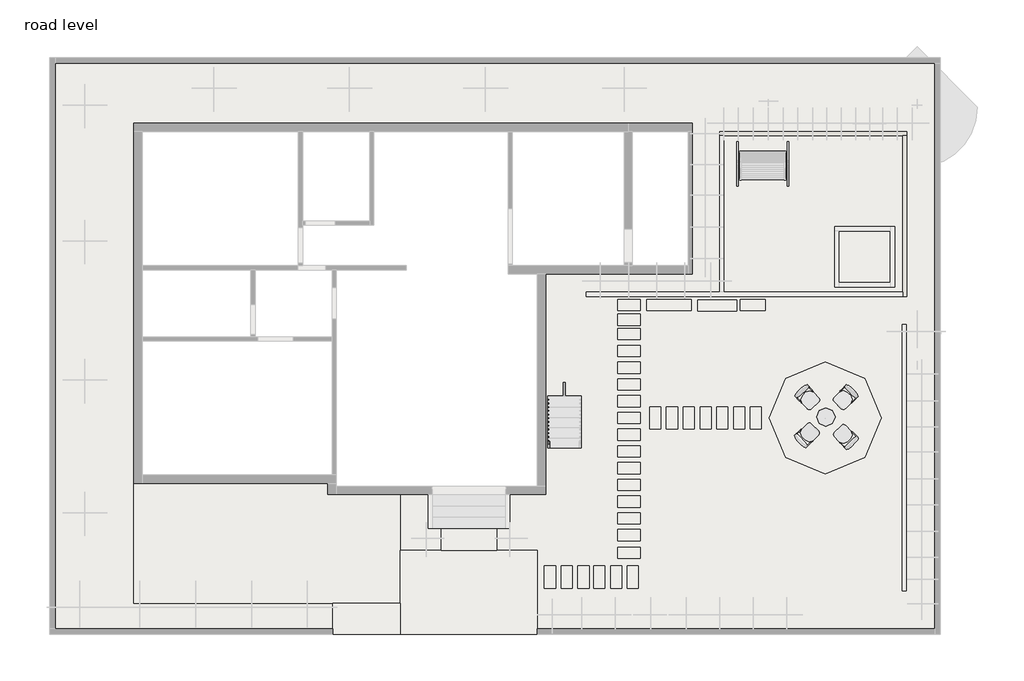
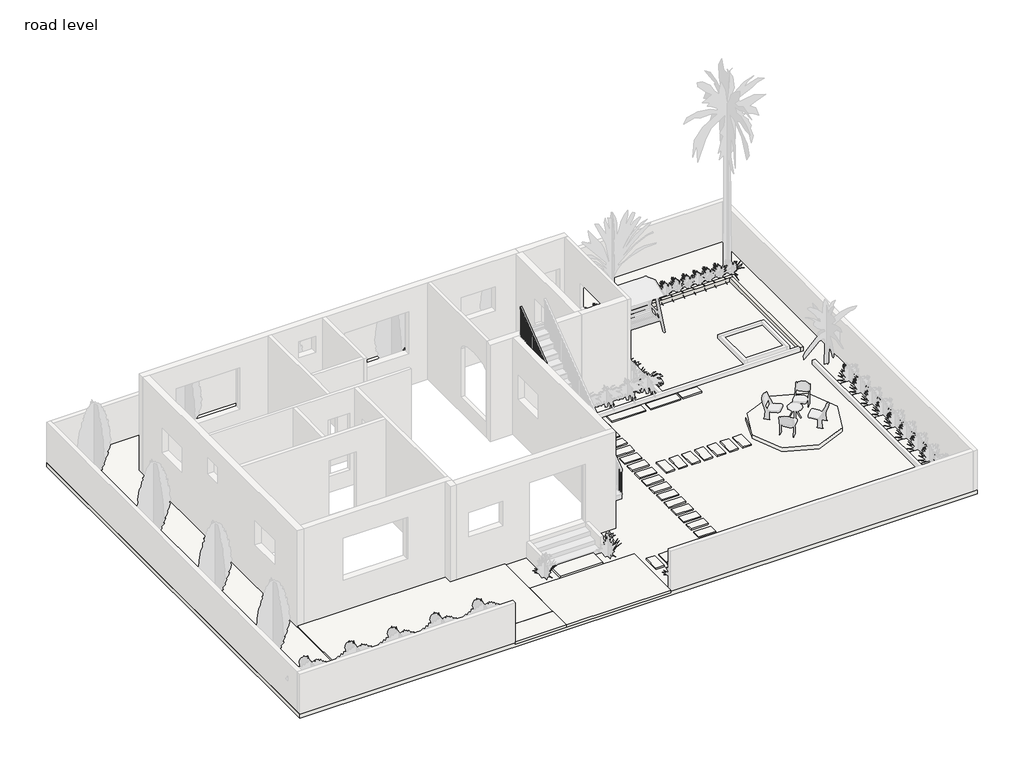
# One storey, part 2 of 3: 12 slabs, 2 walls, 1 railing.
"""IFC4 building model written with IfcOpenShell, lengths in millimetres."""

from ifc_helpers import new_model, si_unit, point, frame, frame_2d, origin, origin_with_axes, place, context, project, spatial, polyline, circle_curve, trimmed, segment, composite_curve, outline, extrude, faceted_brep, element, save

model = new_model("IFC4")

# Units and contexts
model_context = context("Model", 3, world=origin())
ifc_project = project(units=[si_unit("LENGTHUNIT", "METRE", prefix="MILLI")], contexts=[model_context])

# Site, building, storey
site = spatial("IfcSite", under=ifc_project)
building = spatial("IfcBuilding", under=site)
storey = spatial("IfcBuildingStorey", under=building, Name="road level", Elevation=0.0)

# Railing
placement = place(None, origin())
element("IfcRailing", 1, ObjectType="Handrail - Rectangular", at=placement, inside=storey, context=model_context, shape_type="SweptSolid", body=[
    extrude(outline(polyline([(3730.2992417, 1062.3350139), (3730.2992417, 1126.0666667), (8480.0992417, 4724.4), (8480.0992417, 4660.6683472), (3730.2992417, 1062.3350139)])), frame((-6743.6917413, 0.0, 0.0), z_axis=(1.0, 0.0, 0.0), x_axis=(0.0, 1.0, 0.0)), (0.0, 0.0, 1.0), 50.8),
    extrude(outline(polyline([(8413.4242417, 4610.1569836), (8413.4242417, 3598.3333333), (8394.3742417, 3598.3333333), (8394.3742417, 4595.7251654), (8413.4242417, 4610.1569836)])), frame((-6727.8167413, 0.0, 0.0), z_axis=(1.0, 0.0, 0.0), x_axis=(0.0, 1.0, 0.0)), (0.0, 0.0, 1.0), 19.05),
    extrude(outline(polyline([(8311.8242417, 4533.1872866), (8311.8242417, 3598.3333333), (8292.7742417, 3598.3333333), (8292.7742417, 4518.7554685), (8311.8242417, 4533.1872866)])), frame((-6727.8167413, 0.0, 0.0), z_axis=(1.0, 0.0, 0.0), x_axis=(0.0, 1.0, 0.0)), (0.0, 0.0, 1.0), 19.05),
    extrude(outline(polyline([(8210.2242417, 4456.2175897), (8210.2242417, 3598.3333333), (8191.1742417, 3598.3333333), (8191.1742417, 4441.7857715), (8210.2242417, 4456.2175897)])), frame((-6727.8167413, 0.0, 0.0), z_axis=(1.0, 0.0, 0.0), x_axis=(0.0, 1.0, 0.0)), (0.0, 0.0, 1.0), 19.05),
    extrude(outline(polyline([(8108.6242417, 4379.2478927), (8108.6242417, 3386.6666667), (8089.5742417, 3386.6666667), (8089.5742417, 4364.8160745), (8108.6242417, 4379.2478927)])), frame((-6727.8167413, 0.0, 0.0), z_axis=(1.0, 0.0, 0.0), x_axis=(0.0, 1.0, 0.0)), (0.0, 0.0, 1.0), 19.05),
    extrude(outline(polyline([(8007.0242417, 4302.2781957), (8007.0242417, 3386.6666667), (7987.9742417, 3386.6666667), (7987.9742417, 4287.8463775), (8007.0242417, 4302.2781957)])), frame((-6727.8167413, 0.0, 0.0), z_axis=(1.0, 0.0, 0.0), x_axis=(0.0, 1.0, 0.0)), (0.0, 0.0, 1.0), 19.05),
    extrude(outline(polyline([(7905.4242417, 4225.3084988), (7905.4242417, 3175.0), (7886.3742417, 3175.0), (7886.3742417, 4210.8766806), (7905.4242417, 4225.3084988)])), frame((-6727.8167413, 0.0, 0.0), z_axis=(1.0, 0.0, 0.0), x_axis=(0.0, 1.0, 0.0)), (0.0, 0.0, 1.0), 19.05),
    extrude(outline(polyline([(7803.8242417, 4148.3388018), (7803.8242417, 3175.0), (7784.7742417, 3175.0), (7784.7742417, 4133.9069836), (7803.8242417, 4148.3388018)])), frame((-6727.8167413, 0.0, 0.0), z_axis=(1.0, 0.0, 0.0), x_axis=(0.0, 1.0, 0.0)), (0.0, 0.0, 1.0), 19.05),
    extrude(outline(polyline([(7702.2242417, 4071.3691048), (7702.2242417, 3175.0), (7683.1742417, 3175.0), (7683.1742417, 4056.9372866), (7702.2242417, 4071.3691048)])), frame((-6727.8167413, 0.0, 0.0), z_axis=(1.0, 0.0, 0.0), x_axis=(0.0, 1.0, 0.0)), (0.0, 0.0, 1.0), 19.05),
    extrude(outline(polyline([(7600.6242417, 3994.3994079), (7600.6242417, 2963.3333333), (7581.5742417, 2963.3333333), (7581.5742417, 3979.9675897), (7600.6242417, 3994.3994079)])), frame((-6727.8167413, 0.0, 0.0), z_axis=(1.0, 0.0, 0.0), x_axis=(0.0, 1.0, 0.0)), (0.0, 0.0, 1.0), 19.05),
    extrude(outline(polyline([(7499.0242417, 3917.4297109), (7499.0242417, 2963.3333333), (7479.9742417, 2963.3333333), (7479.9742417, 3902.9978927), (7499.0242417, 3917.4297109)])), frame((-6727.8167413, 0.0, 0.0), z_axis=(1.0, 0.0, 0.0), x_axis=(0.0, 1.0, 0.0)), (0.0, 0.0, 1.0), 19.05),
    extrude(outline(polyline([(7397.4242417, 3840.4600139), (7397.4242417, 2963.3333333), (7378.3742417, 2963.3333333), (7378.3742417, 3826.0281957), (7397.4242417, 3840.4600139)])), frame((-6727.8167413, 0.0, 0.0), z_axis=(1.0, 0.0, 0.0), x_axis=(0.0, 1.0, 0.0)), (0.0, 0.0, 1.0), 19.05),
    extrude(outline(polyline([(7295.8242417, 3763.4903169), (7295.8242417, 2751.6666667), (7276.7742417, 2751.6666667), (7276.7742417, 3749.0584988), (7295.8242417, 3763.4903169)])), frame((-6727.8167413, 0.0, 0.0), z_axis=(1.0, 0.0, 0.0), x_axis=(0.0, 1.0, 0.0)), (0.0, 0.0, 1.0), 19.05),
    extrude(outline(polyline([(7194.2242417, 3686.52062), (7194.2242417, 2751.6666667), (7175.1742417, 2751.6666667), (7175.1742417, 3672.0888018), (7194.2242417, 3686.52062)])), frame((-6727.8167413, 0.0, 0.0), z_axis=(1.0, 0.0, 0.0), x_axis=(0.0, 1.0, 0.0)), (0.0, 0.0, 1.0), 19.05),
    extrude(outline(polyline([(7092.6242417, 3609.550923), (7092.6242417, 2751.6666667), (7073.5742417, 2751.6666667), (7073.5742417, 3595.1191048), (7092.6242417, 3609.550923)])), frame((-6727.8167413, 0.0, 0.0), z_axis=(1.0, 0.0, 0.0), x_axis=(0.0, 1.0, 0.0)), (0.0, 0.0, 1.0), 19.05),
    extrude(outline(polyline([(6991.0242417, 3532.581226), (6991.0242417, 2540.0), (6971.9742417, 2540.0), (6971.9742417, 3518.1494079), (6991.0242417, 3532.581226)])), frame((-6727.8167413, 0.0, 0.0), z_axis=(1.0, 0.0, 0.0), x_axis=(0.0, 1.0, 0.0)), (0.0, 0.0, 1.0), 19.05),
    extrude(outline(polyline([(6889.4242417, 3455.6115291), (6889.4242417, 2540.0), (6870.3742417, 2540.0), (6870.3742417, 3441.1797109), (6889.4242417, 3455.6115291)])), frame((-6727.8167413, 0.0, 0.0), z_axis=(1.0, 0.0, 0.0), x_axis=(0.0, 1.0, 0.0)), (0.0, 0.0, 1.0), 19.05),
    extrude(outline(polyline([(6787.8242417, 3378.6418321), (6787.8242417, 2328.3333333), (6768.7742417, 2328.3333333), (6768.7742417, 3364.2100139), (6787.8242417, 3378.6418321)])), frame((-6727.8167413, 0.0, 0.0), z_axis=(1.0, 0.0, 0.0), x_axis=(0.0, 1.0, 0.0)), (0.0, 0.0, 1.0), 19.05),
    extrude(outline(polyline([(6686.2242417, 3301.6721351), (6686.2242417, 2328.3333333), (6667.1742417, 2328.3333333), (6667.1742417, 3287.2403169), (6686.2242417, 3301.6721351)])), frame((-6727.8167413, 0.0, 0.0), z_axis=(1.0, 0.0, 0.0), x_axis=(0.0, 1.0, 0.0)), (0.0, 0.0, 1.0), 19.05),
    extrude(outline(polyline([(6584.6242417, 3224.7024382), (6584.6242417, 2328.3333333), (6565.5742417, 2328.3333333), (6565.5742417, 3210.27062), (6584.6242417, 3224.7024382)])), frame((-6727.8167413, 0.0, 0.0), z_axis=(1.0, 0.0, 0.0), x_axis=(0.0, 1.0, 0.0)), (0.0, 0.0, 1.0), 19.05),
    extrude(outline(polyline([(6483.0242417, 3147.7327412), (6483.0242417, 2116.6666667), (6463.9742417, 2116.6666667), (6463.9742417, 3133.300923), (6483.0242417, 3147.7327412)])), frame((-6727.8167413, 0.0, 0.0), z_axis=(1.0, 0.0, 0.0), x_axis=(0.0, 1.0, 0.0)), (0.0, 0.0, 1.0), 19.05),
    extrude(outline(polyline([(6381.4242417, 3070.7630442), (6381.4242417, 2116.6666667), (6362.3742417, 2116.6666667), (6362.3742417, 3056.331226), (6381.4242417, 3070.7630442)])), frame((-6727.8167413, 0.0, 0.0), z_axis=(1.0, 0.0, 0.0), x_axis=(0.0, 1.0, 0.0)), (0.0, 0.0, 1.0), 19.05),
    extrude(outline(polyline([(6279.8242417, 2993.7933472), (6279.8242417, 2116.6666667), (6260.7742417, 2116.6666667), (6260.7742417, 2979.3615291), (6279.8242417, 2993.7933472)])), frame((-6727.8167413, 0.0, 0.0), z_axis=(1.0, 0.0, 0.0), x_axis=(0.0, 1.0, 0.0)), (0.0, 0.0, 1.0), 19.05),
    extrude(outline(polyline([(6178.2242417, 2916.8236503), (6178.2242417, 1905.0), (6159.1742417, 1905.0), (6159.1742417, 2902.3918321), (6178.2242417, 2916.8236503)])), frame((-6727.8167413, 0.0, 0.0), z_axis=(1.0, 0.0, 0.0), x_axis=(0.0, 1.0, 0.0)), (0.0, 0.0, 1.0), 19.05),
    extrude(outline(polyline([(6076.6242417, 2839.8539533), (6076.6242417, 1905.0), (6057.5742417, 1905.0), (6057.5742417, 2825.4221351), (6076.6242417, 2839.8539533)])), frame((-6727.8167413, 0.0, 0.0), z_axis=(1.0, 0.0, 0.0), x_axis=(0.0, 1.0, 0.0)), (0.0, 0.0, 1.0), 19.05),
    extrude(outline(polyline([(5975.0242417, 2762.8842563), (5975.0242417, 1905.0), (5955.9742417, 1905.0), (5955.9742417, 2748.4524382), (5975.0242417, 2762.8842563)])), frame((-6727.8167413, 0.0, 0.0), z_axis=(1.0, 0.0, 0.0), x_axis=(0.0, 1.0, 0.0)), (0.0, 0.0, 1.0), 19.05),
    extrude(outline(polyline([(5873.4242417, 2685.9145594), (5873.4242417, 1693.3333333), (5854.3742417, 1693.3333333), (5854.3742417, 2671.4827412), (5873.4242417, 2685.9145594)])), frame((-6727.8167413, 0.0, 0.0), z_axis=(1.0, 0.0, 0.0), x_axis=(0.0, 1.0, 0.0)), (0.0, 0.0, 1.0), 19.05),
    extrude(outline(polyline([(5771.8242417, 2608.9448624), (5771.8242417, 1693.3333333), (5752.7742417, 1693.3333333), (5752.7742417, 2594.5130442), (5771.8242417, 2608.9448624)])), frame((-6727.8167413, 0.0, 0.0), z_axis=(1.0, 0.0, 0.0), x_axis=(0.0, 1.0, 0.0)), (0.0, 0.0, 1.0), 19.05),
    extrude(outline(polyline([(5670.2242417, 2531.9751654), (5670.2242417, 1481.6666667), (5651.1742417, 1481.6666667), (5651.1742417, 2517.5433472), (5670.2242417, 2531.9751654)])), frame((-6727.8167413, 0.0, 0.0), z_axis=(1.0, 0.0, 0.0), x_axis=(0.0, 1.0, 0.0)), (0.0, 0.0, 1.0), 19.05),
    extrude(outline(polyline([(5568.6242417, 2455.0054685), (5568.6242417, 1481.6666667), (5549.5742417, 1481.6666667), (5549.5742417, 2440.5736503), (5568.6242417, 2455.0054685)])), frame((-6727.8167413, 0.0, 0.0), z_axis=(1.0, 0.0, 0.0), x_axis=(0.0, 1.0, 0.0)), (0.0, 0.0, 1.0), 19.05),
    extrude(outline(polyline([(5467.0242417, 2378.0357715), (5467.0242417, 1481.6666667), (5447.9742417, 1481.6666667), (5447.9742417, 2363.6039533), (5467.0242417, 2378.0357715)])), frame((-6727.8167413, 0.0, 0.0), z_axis=(1.0, 0.0, 0.0), x_axis=(0.0, 1.0, 0.0)), (0.0, 0.0, 1.0), 19.05),
    extrude(outline(polyline([(5365.4242417, 2301.0660745), (5365.4242417, 1270.0), (5346.3742417, 1270.0), (5346.3742417, 2286.6342563), (5365.4242417, 2301.0660745)])), frame((-6727.8167413, 0.0, 0.0), z_axis=(1.0, 0.0, 0.0), x_axis=(0.0, 1.0, 0.0)), (0.0, 0.0, 1.0), 19.05),
    extrude(outline(polyline([(5263.8242417, 2224.0963775), (5263.8242417, 1270.0), (5244.7742417, 1270.0), (5244.7742417, 2209.6645594), (5263.8242417, 2224.0963775)])), frame((-6727.8167413, 0.0, 0.0), z_axis=(1.0, 0.0, 0.0), x_axis=(0.0, 1.0, 0.0)), (0.0, 0.0, 1.0), 19.05),
    extrude(outline(polyline([(5162.2242417, 2147.1266806), (5162.2242417, 1270.0), (5143.1742417, 1270.0), (5143.1742417, 2132.6948624), (5162.2242417, 2147.1266806)])), frame((-6727.8167413, 0.0, 0.0), z_axis=(1.0, 0.0, 0.0), x_axis=(0.0, 1.0, 0.0)), (0.0, 0.0, 1.0), 19.05),
    extrude(outline(polyline([(5060.6242417, 2070.1569836), (5060.6242417, 1058.3333333), (5041.5742417, 1058.3333333), (5041.5742417, 2055.7251654), (5060.6242417, 2070.1569836)])), frame((-6727.8167413, 0.0, 0.0), z_axis=(1.0, 0.0, 0.0), x_axis=(0.0, 1.0, 0.0)), (0.0, 0.0, 1.0), 19.05),
    extrude(outline(polyline([(4959.0242417, 1993.1872866), (4959.0242417, 1058.3333333), (4939.9742417, 1058.3333333), (4939.9742417, 1978.7554685), (4959.0242417, 1993.1872866)])), frame((-6727.8167413, 0.0, 0.0), z_axis=(1.0, 0.0, 0.0), x_axis=(0.0, 1.0, 0.0)), (0.0, 0.0, 1.0), 19.05),
    extrude(outline(polyline([(4857.4242417, 1916.2175897), (4857.4242417, 1058.3333333), (4838.3742417, 1058.3333333), (4838.3742417, 1901.7857715), (4857.4242417, 1916.2175897)])), frame((-6727.8167413, 0.0, 0.0), z_axis=(1.0, 0.0, 0.0), x_axis=(0.0, 1.0, 0.0)), (0.0, 0.0, 1.0), 19.05),
    extrude(outline(polyline([(4755.8242417, 1839.2478927), (4755.8242417, 846.6666667), (4736.7742417, 846.6666667), (4736.7742417, 1824.8160745), (4755.8242417, 1839.2478927)])), frame((-6727.8167413, 0.0, 0.0), z_axis=(1.0, 0.0, 0.0), x_axis=(0.0, 1.0, 0.0)), (0.0, 0.0, 1.0), 19.05),
    extrude(outline(polyline([(4654.2242417, 1762.2781957), (4654.2242417, 846.6666667), (4635.1742417, 846.6666667), (4635.1742417, 1747.8463775), (4654.2242417, 1762.2781957)])), frame((-6727.8167413, 0.0, 0.0), z_axis=(1.0, 0.0, 0.0), x_axis=(0.0, 1.0, 0.0)), (0.0, 0.0, 1.0), 19.05),
    extrude(outline(polyline([(4552.6242417, 1685.3084988), (4552.6242417, 635.0), (4533.5742417, 635.0), (4533.5742417, 1670.8766806), (4552.6242417, 1685.3084988)])), frame((-6727.8167413, 0.0, 0.0), z_axis=(1.0, 0.0, 0.0), x_axis=(0.0, 1.0, 0.0)), (0.0, 0.0, 1.0), 19.05),
    extrude(outline(polyline([(4451.0242417, 1608.3388018), (4451.0242417, 635.0), (4431.9742417, 635.0), (4431.9742417, 1593.9069836), (4451.0242417, 1608.3388018)])), frame((-6727.8167413, 0.0, 0.0), z_axis=(1.0, 0.0, 0.0), x_axis=(0.0, 1.0, 0.0)), (0.0, 0.0, 1.0), 19.05),
    extrude(outline(polyline([(4349.4242417, 1531.3691048), (4349.4242417, 635.0), (4330.3742417, 635.0), (4330.3742417, 1516.9372866), (4349.4242417, 1531.3691048)])), frame((-6727.8167413, 0.0, 0.0), z_axis=(1.0, 0.0, 0.0), x_axis=(0.0, 1.0, 0.0)), (0.0, 0.0, 1.0), 19.05),
    extrude(outline(polyline([(4247.8242417, 1454.3994079), (4247.8242417, 423.3333333), (4228.7742417, 423.3333333), (4228.7742417, 1439.9675897), (4247.8242417, 1454.3994079)])), frame((-6727.8167413, 0.0, 0.0), z_axis=(1.0, 0.0, 0.0), x_axis=(0.0, 1.0, 0.0)), (0.0, 0.0, 1.0), 19.05),
    extrude(outline(polyline([(4146.2242417, 1377.4297109), (4146.2242417, 423.3333333), (4127.1742417, 423.3333333), (4127.1742417, 1362.9978927), (4146.2242417, 1377.4297109)])), frame((-6727.8167413, 0.0, 0.0), z_axis=(1.0, 0.0, 0.0), x_axis=(0.0, 1.0, 0.0)), (0.0, 0.0, 1.0), 19.05),
    extrude(outline(polyline([(4044.6242417, 1300.4600139), (4044.6242417, 423.3333333), (4025.5742417, 423.3333333), (4025.5742417, 1286.0281957), (4044.6242417, 1300.4600139)])), frame((-6727.8167413, 0.0, 0.0), z_axis=(1.0, 0.0, 0.0), x_axis=(0.0, 1.0, 0.0)), (0.0, 0.0, 1.0), 19.05),
    extrude(outline(polyline([(3943.0242417, 1223.4903169), (3943.0242417, 211.6666667), (3923.9742417, 211.6666667), (3923.9742417, 1209.0584988), (3943.0242417, 1223.4903169)])), frame((-6727.8167413, 0.0, 0.0), z_axis=(1.0, 0.0, 0.0), x_axis=(0.0, 1.0, 0.0)), (0.0, 0.0, 1.0), 19.05),
    extrude(outline(polyline([(3841.4242417, 1146.52062), (3841.4242417, 211.6666667), (3822.3742417, 211.6666667), (3822.3742417, 1132.0888018), (3841.4242417, 1146.52062)])), frame((-6727.8167413, 0.0, 0.0), z_axis=(1.0, 0.0, 0.0), x_axis=(0.0, 1.0, 0.0)), (0.0, 0.0, 1.0), 19.05),
    extrude(outline(polyline([(8480.0992417, 4660.6683472), (8480.0992417, 3598.3333333), (8461.0492417, 3598.3333333), (8461.0492417, 4646.2365291), (8480.0992417, 4660.6683472)])), frame((-6727.8167413, 0.0, 0.0), z_axis=(1.0, 0.0, 0.0), x_axis=(0.0, 1.0, 0.0)), (0.0, 0.0, 1.0), 19.05),
    extrude(outline(polyline([(3749.3492417, 1076.7668321), (3749.3492417, 211.6666667), (3730.2992417, 211.6666667), (3730.2992417, 1062.3350139), (3749.3492417, 1076.7668321)])), frame((-6727.8167413, 0.0, 0.0), z_axis=(1.0, 0.0, 0.0), x_axis=(0.0, 1.0, 0.0)), (0.0, 0.0, 1.0), 19.05),
])

# Slabs
element("IfcSlab", 2, ObjectType="Generic - 2", at=placement, inside=storey, context=model_context, shape_type="SweptSolid", body=[
    extrude(outline(polyline([(2605.0138793, 9654.4970238), (2605.0138793, 8244.7970238), (1195.3138793, 8244.7970238), (1195.3138793, 9654.4970238), (2605.0138793, 9654.4970238)])), origin_with_axes(), (0.0, 0.0, 1.0), 50.8),
])
element("IfcSlab", 3, ObjectType="Generic - 2\" 2", at=placement, inside=storey, context=model_context, shape_type="SweptSolid", body=[
    extrude(outline(polyline([(-4216.3917413, 7786.7980818), (-4216.3917413, 7481.9980818), (-4825.9917413, 7481.9980818), (-4825.9917413, 7786.7980818), (-4216.3917413, 7786.7980818)])), frame((0.0, 0.0, -50.8), z_axis=(0.0, 0.0, 1.0), x_axis=(1.0, 0.0, 0.0)), (0.0, 0.0, 1.0), 101.6),
])
element("IfcSlab", 4, ObjectType="Generic - 2\" 2", at=placement, inside=storey, context=model_context, shape_type="SweptSolid", body=[
    extrude(outline(polyline([(-2824.9924466, 7783.876947), (-2824.9924466, 7479.076947), (-4044.1924466, 7479.076947), (-4044.1924466, 7783.876947), (-2824.9924466, 7783.876947)])), frame((0.0, 0.0, -50.8), z_axis=(0.0, 0.0, 1.0), x_axis=(1.0, 0.0, 0.0)), (0.0, 0.0, 1.0), 101.6),
    extrude(outline(polyline([(-815.4995339, 7783.876947), (-815.4995339, 7479.076947), (-1495.8466995, 7479.076947), (-1495.8466995, 7783.876947), (-815.4995339, 7783.876947)])), frame((0.0, 0.0, -50.8), z_axis=(0.0, 0.0, 1.0), x_axis=(1.0, 0.0, 0.0)), (0.0, 0.0, 1.0), 101.6),
])
element("IfcSlab", 5, ObjectType="Generic - 2\" 3", at=placement, inside=storey, context=model_context, shape_type="SweptSolid", body=[
    extrude(outline(polyline([(-1583.8375852, 7774.2549493), (-1583.8375852, 7469.4549493), (-2650.6375852, 7469.4549493), (-2650.6375852, 7774.2549493), (-1583.8375852, 7774.2549493)])), frame((0.0, 0.0, -50.8), z_axis=(0.0, 0.0, 1.0), x_axis=(1.0, 0.0, 0.0)), (0.0, 0.0, 1.0), 101.6),
    extrude(outline(polyline([(-4216.3917413, 7382.2968487), (-4216.3917413, 7077.4968487), (-4825.9917413, 7077.4968487), (-4825.9917413, 7382.2968487), (-4216.3917413, 7382.2968487)])), frame((0.0, 0.0, -50.8), z_axis=(0.0, 0.0, 1.0), x_axis=(1.0, 0.0, 0.0)), (0.0, 0.0, 1.0), 101.6),
])
element("IfcSlab", 6, ObjectType="Generic - 2\" 4", at=placement, inside=storey, context=model_context, shape_type="SweptSolid", body=[
    extrude(outline(polyline([(-4216.3917413, 6991.9811291), (-4216.3917413, 6687.1811291), (-4825.9917413, 6687.1811291), (-4825.9917413, 6991.9811291), (-4216.3917413, 6991.9811291)])), frame((0.0, 0.0, -50.8), z_axis=(0.0, 0.0, 1.0), x_axis=(1.0, 0.0, 0.0)), (0.0, 0.0, 1.0), 101.6),
    extrude(outline(polyline([(-4216.3917413, 6534.7811291), (-4216.3917413, 6229.9811291), (-4825.9917413, 6229.9811291), (-4825.9917413, 6534.7811291), (-4216.3917413, 6534.7811291)])), frame((0.0, 0.0, -50.8), z_axis=(0.0, 0.0, 1.0), x_axis=(1.0, 0.0, 0.0)), (0.0, 0.0, 1.0), 101.6),
    extrude(outline(polyline([(-4216.3917413, 6077.5811291), (-4216.3917413, 5772.7811291), (-4825.9917413, 5772.7811291), (-4825.9917413, 6077.5811291), (-4216.3917413, 6077.5811291)])), frame((0.0, 0.0, -50.8), z_axis=(0.0, 0.0, 1.0), x_axis=(1.0, 0.0, 0.0)), (0.0, 0.0, 1.0), 101.6),
    extrude(outline(polyline([(-4216.3917413, 5620.3811291), (-4216.3917413, 5315.5811291), (-4825.9917413, 5315.5811291), (-4825.9917413, 5620.3811291), (-4216.3917413, 5620.3811291)])), frame((0.0, 0.0, -50.8), z_axis=(0.0, 0.0, 1.0), x_axis=(1.0, 0.0, 0.0)), (0.0, 0.0, 1.0), 101.6),
    extrude(outline(polyline([(-4216.3917413, 5163.1811291), (-4216.3917413, 4858.3811291), (-4825.9917413, 4858.3811291), (-4825.9917413, 5163.1811291), (-4216.3917413, 5163.1811291)])), frame((0.0, 0.0, -50.8), z_axis=(0.0, 0.0, 1.0), x_axis=(1.0, 0.0, 0.0)), (0.0, 0.0, 1.0), 101.6),
    extrude(outline(polyline([(-4216.3917413, 4705.9811291), (-4216.3917413, 4401.1811291), (-4825.9917413, 4401.1811291), (-4825.9917413, 4705.9811291), (-4216.3917413, 4705.9811291)])), frame((0.0, 0.0, -50.8), z_axis=(0.0, 0.0, 1.0), x_axis=(1.0, 0.0, 0.0)), (0.0, 0.0, 1.0), 101.6),
    extrude(outline(polyline([(-4216.3917413, 4248.7811291), (-4216.3917413, 3943.9811291), (-4825.9917413, 3943.9811291), (-4825.9917413, 4248.7811291), (-4216.3917413, 4248.7811291)])), frame((0.0, 0.0, -50.8), z_axis=(0.0, 0.0, 1.0), x_axis=(1.0, 0.0, 0.0)), (0.0, 0.0, 1.0), 101.6),
    extrude(outline(polyline([(-4216.3917413, 3791.5811291), (-4216.3917413, 3486.7811291), (-4825.9917413, 3486.7811291), (-4825.9917413, 3791.5811291), (-4216.3917413, 3791.5811291)])), frame((0.0, 0.0, -50.8), z_axis=(0.0, 0.0, 1.0), x_axis=(1.0, 0.0, 0.0)), (0.0, 0.0, 1.0), 101.6),
    extrude(outline(polyline([(-4216.3917413, 3334.3811291), (-4216.3917413, 3029.5811291), (-4825.9917413, 3029.5811291), (-4825.9917413, 3334.3811291), (-4216.3917413, 3334.3811291)])), frame((0.0, 0.0, -50.8), z_axis=(0.0, 0.0, 1.0), x_axis=(1.0, 0.0, 0.0)), (0.0, 0.0, 1.0), 101.6),
    extrude(outline(polyline([(-4216.3917413, 2877.1811291), (-4216.3917413, 2572.3811291), (-4825.9917413, 2572.3811291), (-4825.9917413, 2877.1811291), (-4216.3917413, 2877.1811291)])), frame((0.0, 0.0, -50.8), z_axis=(0.0, 0.0, 1.0), x_axis=(1.0, 0.0, 0.0)), (0.0, 0.0, 1.0), 101.6),
    extrude(outline(polyline([(-4216.3917413, 2419.9811291), (-4216.3917413, 2115.1811291), (-4825.9917413, 2115.1811291), (-4825.9917413, 2419.9811291), (-4216.3917413, 2419.9811291)])), frame((0.0, 0.0, -50.8), z_axis=(0.0, 0.0, 1.0), x_axis=(1.0, 0.0, 0.0)), (0.0, 0.0, 1.0), 101.6),
    extrude(outline(polyline([(-4216.3917413, 1962.7811291), (-4216.3917413, 1657.9811291), (-4825.9917413, 1657.9811291), (-4825.9917413, 1962.7811291), (-4216.3917413, 1962.7811291)])), frame((0.0, 0.0, -50.8), z_axis=(0.0, 0.0, 1.0), x_axis=(1.0, 0.0, 0.0)), (0.0, 0.0, 1.0), 101.6),
    extrude(outline(polyline([(-4216.3917413, 1505.5811291), (-4216.3917413, 1200.7811291), (-4825.9917413, 1200.7811291), (-4825.9917413, 1505.5811291), (-4216.3917413, 1505.5811291)])), frame((0.0, 0.0, -50.8), z_axis=(0.0, 0.0, 1.0), x_axis=(1.0, 0.0, 0.0)), (0.0, 0.0, 1.0), 101.6),
    extrude(outline(polyline([(-6527.7917413, -94.6188709), (-6832.5917413, -94.6188709), (-6832.5917413, 514.9811291), (-6527.7917413, 514.9811291), (-6527.7917413, -94.6188709)])), frame((0.0, 0.0, -50.8), z_axis=(0.0, 0.0, 1.0), x_axis=(1.0, 0.0, 0.0)), (0.0, 0.0, 1.0), 101.6),
    extrude(outline(polyline([(-6070.5917413, -94.6188709), (-6375.3917413, -94.6188709), (-6375.3917413, 514.9811291), (-6070.5917413, 514.9811291), (-6070.5917413, -94.6188709)])), frame((0.0, 0.0, -50.8), z_axis=(0.0, 0.0, 1.0), x_axis=(1.0, 0.0, 0.0)), (0.0, 0.0, 1.0), 101.6),
    extrude(outline(polyline([(-5613.3917413, -94.6188709), (-5918.1917413, -94.6188709), (-5918.1917413, 514.9811291), (-5613.3917413, 514.9811291), (-5613.3917413, -94.6188709)])), frame((0.0, 0.0, -50.8), z_axis=(0.0, 0.0, 1.0), x_axis=(1.0, 0.0, 0.0)), (0.0, 0.0, 1.0), 101.6),
    extrude(outline(polyline([(-4216.3917413, 1022.9811291), (-4216.3917413, 718.1811291), (-4825.9917413, 718.1811291), (-4825.9917413, 1022.9811291), (-4216.3917413, 1022.9811291)])), frame((0.0, 0.0, -50.8), z_axis=(0.0, 0.0, 1.0), x_axis=(1.0, 0.0, 0.0)), (0.0, 0.0, 1.0), 101.6),
    extrude(outline(polyline([(-912.286018, 4248.7811291), (-1217.086018, 4248.7811291), (-1217.086018, 4858.3811291), (-912.286018, 4858.3811291), (-912.286018, 4248.7811291)])), frame((0.0, 0.0, -50.8), z_axis=(0.0, 0.0, 1.0), x_axis=(1.0, 0.0, 0.0)), (0.0, 0.0, 1.0), 101.6),
    extrude(outline(polyline([(-1369.486018, 4248.7811291), (-1674.286018, 4248.7811291), (-1674.286018, 4858.3811291), (-1369.486018, 4858.3811291), (-1369.486018, 4248.7811291)])), frame((0.0, 0.0, -50.8), z_axis=(0.0, 0.0, 1.0), x_axis=(1.0, 0.0, 0.0)), (0.0, 0.0, 1.0), 101.6),
    extrude(outline(polyline([(-1826.686018, 4248.7811291), (-2131.486018, 4248.7811291), (-2131.486018, 4858.3811291), (-1826.686018, 4858.3811291), (-1826.686018, 4248.7811291)])), frame((0.0, 0.0, -50.8), z_axis=(0.0, 0.0, 1.0), x_axis=(1.0, 0.0, 0.0)), (0.0, 0.0, 1.0), 101.6),
    extrude(outline(polyline([(-2283.886018, 4248.7811291), (-2588.686018, 4248.7811291), (-2588.686018, 4858.3811291), (-2283.886018, 4858.3811291), (-2283.886018, 4248.7811291)])), frame((0.0, 0.0, -50.8), z_axis=(0.0, 0.0, 1.0), x_axis=(1.0, 0.0, 0.0)), (0.0, 0.0, 1.0), 101.6),
    extrude(outline(polyline([(-2741.086018, 4248.7811291), (-3045.886018, 4248.7811291), (-3045.886018, 4858.3811291), (-2741.086018, 4858.3811291), (-2741.086018, 4248.7811291)])), frame((0.0, 0.0, -50.8), z_axis=(0.0, 0.0, 1.0), x_axis=(1.0, 0.0, 0.0)), (0.0, 0.0, 1.0), 101.6),
    extrude(outline(polyline([(-3198.286018, 4248.7811291), (-3503.086018, 4248.7811291), (-3503.086018, 4858.3811291), (-3198.286018, 4858.3811291), (-3198.286018, 4248.7811291)])), frame((0.0, 0.0, -50.8), z_axis=(0.0, 0.0, 1.0), x_axis=(1.0, 0.0, 0.0)), (0.0, 0.0, 1.0), 101.6),
    extrude(outline(polyline([(-3655.486018, 4248.7811291), (-3960.286018, 4248.7811291), (-3960.286018, 4858.3811291), (-3655.486018, 4858.3811291), (-3655.486018, 4248.7811291)])), frame((0.0, 0.0, -50.8), z_axis=(0.0, 0.0, 1.0), x_axis=(1.0, 0.0, 0.0)), (0.0, 0.0, 1.0), 101.6),
    extrude(outline(polyline([(-5181.5917413, -94.6188709), (-5486.3917413, -94.6188709), (-5486.3917413, 514.9811291), (-5181.5917413, 514.9811291), (-5181.5917413, -94.6188709)])), frame((0.0, 0.0, -50.8), z_axis=(0.0, 0.0, 1.0), x_axis=(1.0, 0.0, 0.0)), (0.0, 0.0, 1.0), 101.6),
    extrude(outline(polyline([(-4724.3917413, -94.6188709), (-5029.1917413, -94.6188709), (-5029.1917413, 514.9811291), (-4724.3917413, 514.9811291), (-4724.3917413, -94.6188709)])), frame((0.0, 0.0, -50.8), z_axis=(0.0, 0.0, 1.0), x_axis=(1.0, 0.0, 0.0)), (0.0, 0.0, 1.0), 101.6),
    extrude(outline(polyline([(-4267.1917413, -94.6188709), (-4571.9917413, -94.6188709), (-4571.9917413, 514.9811291), (-4267.1917413, 514.9811291), (-4267.1917413, -94.6188709)])), frame((0.0, 0.0, -50.8), z_axis=(0.0, 0.0, 1.0), x_axis=(1.0, 0.0, 0.0)), (0.0, 0.0, 1.0), 101.6),
])
element("IfcSlab", 7, ObjectType="Generic - 2\" 5", at=placement, inside=storey, context=model_context, shape_type="SweptSolid", body=[
    extrude(outline(polyline([(-18033.9917413, -511.8034782), (-18033.9917413, 2764.7965218), (-12738.0917413, 2764.7965218), (-12738.0917413, 2459.9965218), (-10769.5917413, 2459.9965218), (-10769.5917413, -511.8034782), (-18033.9917413, -511.8034782)])), frame((0.0, 0.0, -50.8), z_axis=(0.0, 0.0, 1.0), x_axis=(1.0, 0.0, 0.0)), (0.0, 0.0, 1.0), 101.6),
])
element("IfcSlab", 8, ObjectType="Generic - 2\" 6", at=placement, inside=storey, context=model_context, shape_type="SweptSolid", body=[
    extrude(outline(polyline([(-10769.5917413, -1350.0034782), (-10769.5917413, 935.9965218), (-7023.0917413, 935.9965218), (-7023.0917413, -1350.0034782), (-10769.5917413, -1350.0034782)])), frame((0.0, 0.0, -50.8), z_axis=(0.0, 0.0, 1.0), x_axis=(1.0, 0.0, 0.0)), (0.0, 0.0, 1.0), 101.6),
])
element("IfcSlab", 9, ObjectType="Generic - 2\" 7", at=placement, inside=storey, context=model_context, shape_type="SweptSolid", body=[
    extrude(outline(polyline([(-12598.3917413, -511.8034782), (-10769.5917413, -511.8034782), (-10769.5917413, -1350.0034782), (-12598.3917413, -1350.0034782), (-12598.3917413, -511.8034782)])), frame((0.0, 0.0, -50.8), z_axis=(0.0, 0.0, 1.0), x_axis=(1.0, 0.0, 0.0)), (0.0, 0.0, 1.0), 101.6),
])
element("IfcSlab", 10, ObjectType="Generic - 4\"", at=placement, inside=storey, context=model_context, shape_type="SweptSolid", body=[
    extrude(outline(polyline([(-9642.3417413, 935.9965218), (-9642.3417413, 1545.5965218), (-8136.2483292, 1545.5965218), (-8136.2483292, 935.9965218), (-9642.3417413, 935.9965218)])), frame((0.0, 0.0, -50.8), z_axis=(0.0, 0.0, 1.0), x_axis=(1.0, 0.0, 0.0)), (0.0, 0.0, 1.0), 152.4),
])
element("IfcSlab", 11, ObjectType="Generic - 6\" 3", at=placement, inside=storey, context=model_context, shape_type="SweptSolid", body=[
    extrude(outline(polyline([(2940.0582587, 12251.6965218), (2940.0582587, 7984.4965218), (-1936.7417413, 7984.4965218), (-1936.7417413, 12251.6965218), (2940.0582587, 12251.6965218)])), frame((0.0, 0.0, -152.4), z_axis=(0.0, 0.0, 1.0), x_axis=(1.0, 0.0, 0.0)), (0.0, 0.0, 1.0), 152.4),
])
element("IfcSlab", 12, ObjectType="Generic - 6\" 4", at=placement, inside=storey, context=model_context, shape_type="SweptSolid", body=[
    extrude(outline(polyline([(3968.7582587, 14385.2965218), (3968.7582587, -1350.0034782), (-20319.9917413, -1350.0034782), (-20319.9917413, 14385.2965218), (3968.7582587, 14385.2965218)]), holes=[polyline([(-2793.9917413, 12594.5965218), (-18033.9917413, 12594.5965218), (-18033.9917413, 2764.7965218), (-12738.0917413, 2764.7965218), (-12738.0917413, 2459.9965218), (-6794.4917413, 2459.9965218), (-6794.4917413, 8479.7965218), (-2793.9917413, 8479.7965218), (-2793.9917413, 12594.5965218)]), polyline([(3054.3582587, 12365.9965218), (-2051.0417413, 12365.9965218), (-2051.0417413, 7870.1965218), (3054.3582587, 7870.1965218), (3054.3582587, 12365.9965218)])]), frame((0.0, 0.0, -152.4), z_axis=(0.0, 0.0, 1.0), x_axis=(1.0, 0.0, 0.0)), (0.0, 0.0, 1.0), 152.4),
])
element("IfcSlab", 13, ObjectType="Generic - 6\" 5", at=placement, inside=storey, context=model_context, shape_type="SweptSolid", body=[
    extrude(outline(composite_curve([segment(trimmed(circle_curve(frame_2d((828.6417041, 4552.6133909)), 1524.0), [point((-695.3582959, 4552.6133909))], [point((2352.6417041, 4552.6133909))], False, "CARTESIAN"), True, "CONTINUOUS"), segment(trimmed(circle_curve(frame_2d((828.6417041, 4552.6133909)), 1524.0), [point((2352.6417041, 4552.6133909))], [point((-695.3582959, 4552.6133909))], False, "CARTESIAN"), True, "CONTINUOUS")], self_intersect=False)), frame((0.0, 0.0, -50.8), z_axis=(0.0, 0.0, 1.0), x_axis=(1.0, 0.0, 0.0)), (0.0, 0.0, 1.0), 203.2),
])

# Walls
element("IfcWall", 14, ObjectType="Generic - 4.5\"", at=placement, inside=storey, context=model_context, shape_type="Brep", body=[
    faceted_brep([(-2051.0417413, 12251.6965218, 0.0), (-1936.7417413, 12251.6965218, 0.0), (2940.0582587, 12251.6965218, 0.0), (3054.3582587, 12251.6965218, 0.0), (3054.3582587, 12251.6965218, 152.4), (2940.0582587, 12251.6965218, 152.4), (-1936.7417413, 12251.6965218, 152.4), (-2051.0417413, 12251.6965218, 152.4), (-2051.0417413, 12365.9965218, 0.0), (-2051.0417413, 12365.9965218, 152.4), (3054.3582587, 12365.9965218, 152.4), (3054.3582587, 12365.9965218, 0.0)], [[[0, 1, 2, 3, 4, 5, 6, 7]], [[8, 9, 10, 11]], [[3, 2, 1, 0, 8, 11]], [[7, 6, 5, 4, 10, 9]], [[4, 3, 11, 10]], [[0, 7, 9, 8]]]),
])
element("IfcWall", 15, ObjectType="Generic - 4.5\"", at=placement, inside=storey, context=model_context, shape_type="Brep", body=[
    faceted_brep([(2940.0582587, 12251.6965218, 0.0), (2940.0582587, 7984.4965218, 0.0), (2940.0582587, 7870.1965218, 0.0), (2940.0582587, 7870.1965218, 152.4), (2940.0582587, 7984.4965218, 152.4), (2940.0582587, 12251.6965218, 152.4), (3054.3582587, 12251.6965218, 0.0), (3054.3582587, 12251.6965218, 152.4), (3054.3582587, 7870.1965218, 152.4), (3054.3582587, 7870.1965218, 0.0)], [[[0, 1, 2, 3, 4, 5]], [[6, 7, 8, 9]], [[2, 1, 0, 6, 9]], [[5, 4, 3, 8, 7]], [[0, 5, 7, 6]], [[3, 2, 9, 8]]]),
])

save(model, "model.ifc")

# Revit data of these elements
# Type "Handrail - Rectangular"
#   Assembly Code = "C2010400"
#   built-in parameter 1008612 = 0.0416667 (stored number, unit not read)
#   built-in parameter 1008611 = 0.0416667 (stored number, unit not read)
#   built-in parameter 1008609 = 0.333333 (stored number, unit not read)
#   built-in parameter 1008604 = 0.166667 (stored number, unit not read)
#   built-in parameter 1008603 = 0.166667 (stored number, unit not read)
#   Railing Height = 3' - 0"
#   built-in parameter 1008630 = 2
#   built-in parameter 1008610 = 2
#   built-in parameter 1008618 = Baluster - Square : 3/4"
# Type "Generic - 2"
#   Assembly Code = "B1010"
#   Function = 0
#   Layers, outside or top first: 0' - 2" "Earth" (function 1)
# Type "Generic - 2\" 2"
#   Assembly Code = "B1010"
#   Function = 0
#   Layers, outside or top first: 0' - 4" "Tile, Mosaic, Gray" (function 1)
# Type "Generic - 2\" 3"
#   Assembly Code = "B1010"
#   Function = 0
#   Layers, outside or top first: 0' - 4" "Tile, Mosaic, Gray" (function 1)
# Type "Generic - 2\" 4"
#   Assembly Code = "B1010"
#   Function = 0
#   Layers, outside or top first: 0' - 4" "Tile, Porcelain, 4in" (function 1)
# Type "Generic - 2\" 5"
#   Assembly Code = "B1010"
#   Function = 0
#   Layers, outside or top first: 0' - 4" "Concrete, Precast" (function 1)
# Type "Generic - 2\" 6"
#   Assembly Code = "B1010"
#   Function = 0
#   Layers, outside or top first: 0' - 4" "Concrete, Precast" (function 1)
# Type "Generic - 2\" 7"
#   Assembly Code = "B1010"
#   Function = 0
#   Layers, outside or top first: 0' - 4" "Concrete, Precast" (function 1)
# Type "Generic - 4\""
#   Assembly Code = "B1010"
#   Function = 0
#   Layers, outside or top first: 0' - 6" "Tile, Mosaic, Gray" (function 1)
# Type "Generic - 6\" 3"
#   Assembly Code = "B1010"
#   Function = 0
#   Layers, outside or top first: 0' - 6" "grass 2" (function 1)
# Type "Generic - 6\" 4"
#   Assembly Code = "B1010"
#   Function = 0
#   Layers, outside or top first: 0' - 6" "Grass" (function 1)
# Type "Generic - 6\" 5"
#   Assembly Code = "B1010"
#   Function = 0
#   Layers, outside or top first: 0' - 8" "Wood Planks" (function 1)
# Type "Generic - 4.5\""
#   Assembly Code = "B2010"
#   Layers, outside or top first: 0' - 4 1/2" no material (function 1)
# Element 1 (IfcRailing, "Handrail - Rectangular")
#   Phase Created = New Construction
# Element 2 (IfcSlab, "Generic - 2")
#   Height Offset From Level = 0' - 2"
#   Phase Created = New Construction
#   Materials on its faces: "Earth"
# Elements 3, 4 (IfcSlab, "Generic - 2\" 2")
#   Height Offset From Level = 0' - 2"
#   Phase Created = New Construction
#   Materials on its faces: "Tile, Mosaic, Gray"
# Element 5 (IfcSlab, "Generic - 2\" 3")
#   Height Offset From Level = 0' - 2"
#   Phase Created = New Construction
#   Materials on its faces: "Tile, Mosaic, Gray"
# Element 6 (IfcSlab, "Generic - 2\" 4")
#   Height Offset From Level = 0' - 2"
#   Phase Created = New Construction
#   Materials on its faces: "Tile, Porcelain, 4in"
# Element 7 (IfcSlab, "Generic - 2\" 5")
#   built-in parameter 1001955 = -1.5708 (stored number, unit not read)
#   Height Offset From Level = 0' - 2"
#   Phase Created = New Construction
#   Materials on its faces: "Concrete, Precast"
# Element 8 (IfcSlab, "Generic - 2\" 6")
#   Height Offset From Level = 0' - 2"
#   Phase Created = New Construction
#   Materials on its faces: "Concrete, Precast"
# Element 9 (IfcSlab, "Generic - 2\" 7")
#   built-in parameter 1001955 = 3.14159 (stored number, unit not read)
#   Height Offset From Level = 0' - 2"
#   Phase Created = New Construction
#   Materials on its faces: "Concrete, Precast"
# Element 10 (IfcSlab, "Generic - 4\"")
#   built-in parameter 1001955 = -1.5708 (stored number, unit not read)
#   Height Offset From Level = 0' - 4"
#   Phase Created = New Construction
#   Materials on its faces: "Tile, Mosaic, Gray"
# Element 11 (IfcSlab, "Generic - 6\" 3")
#   Height Offset From Level = 0' - 0"
#   Phase Created = New Construction
#   Materials on its faces: "grass 2"
# Element 12 (IfcSlab, "Generic - 6\" 4")
#   Height Offset From Level = 0' - 0"
#   Phase Created = New Construction
#   Materials on its faces: "Grass"
# Element 13 (IfcSlab, "Generic - 6\" 5")
#   Height Offset From Level = 0' - 6"
#   Phase Created = New Construction
#   Materials on its faces: "Wood Planks"
# Elements 14, 15 (IfcWall, "Generic - 4.5\"")
#   Top Offset = 0' - 0"
#   Base Offset = 0' - 0"
#   Unconnected Height = 0' - 6"
#   wall height = 0' - 6"
#   Phase Created = New Construction
#   Base Constraint = road level
#   Materials on its faces: "Default Wall"
# Materials
#   "Earth": class "Generic", colour RGB 97 75 62, transparency 0, Description = "Soil", Cost = 0
#   "Tile, Mosaic, Gray": class "Generic", colour RGB 127 127 127, transparency 0, Description = "Mosiac tile, gray", Cost = 0
#   "Tile, Porcelain, 4in": class "Generic", colour RGB 89 87 158, transparency 0, Description = "Porcelain tile, 4\", white", Cost = 0
#   "Concrete, Precast": class "Concrete", colour RGB 198 187 187, transparency 0, Description = "Precast concrete", Cost = 0
#   "grass 2": class "Generic", colour RGB 120 120 120, transparency 0, Cost = 0
#   "Grass": class "Generic", colour RGB 104 137 66, transparency 0, Description = "Physical material.", Cost = 0
#   "Wood Planks": class "Wood", colour RGB 193 160 115, transparency 0, Description = "Physical material.", Cost = 0
#   "Default Wall": colour RGB 128 128 128, transparency 0, Cost = 0
